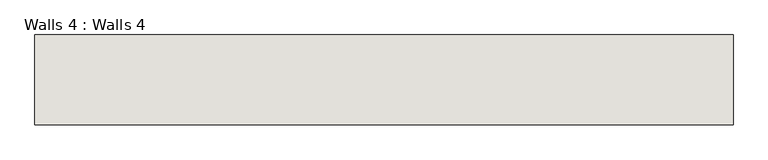
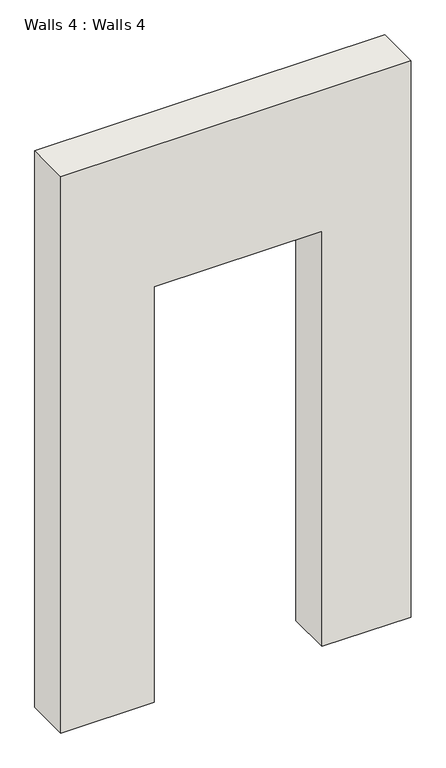
"""IFC4 building model written with IfcOpenShell, lengths in millimetres: wall geometry, Walls 4 : Walls 4."""

from ifc_helpers import new_model, si_unit, frame, origin, place, context, project, spatial, polyline, outline, extrude, source, transform, mapped, element, save


def walls_4_walls_4_cd32183e(model_context):
    return source(origin(), model_context, "Body", "SweptSolid", [
        extrude(outline(polyline([(12109.1166012, -6816.4084212), (12109.1166012, -9490.3075311), (7623.0321664, -9490.3075311), (7623.0321664, -8777.0745124), (10972.8, -8777.0745124), (10972.8, -7495.2589248), (7623.0321664, -7495.2589248), (7623.0321664, -6816.4084212), (12109.1166012, -6816.4084212)])), frame((0.0, -896.8189974, 0.0), z_axis=(0.0, 1.0, 0.0), x_axis=(0.0, 0.0, 1.0)), (0.0, 0.0, 1.0), 344.5607879),
    ])


if __name__ == "__main__":
    model = new_model("IFC4")
    model_context = context("Model", 3, world=origin())
    ifc_project = project(units=[si_unit("LENGTHUNIT", "METRE", prefix="MILLI")], contexts=[model_context])
    site = spatial("IfcSite", under=ifc_project)
    building = spatial("IfcBuilding", under=site)
    placement = place(None, origin())
    walls_4_walls_4_shape = walls_4_walls_4_cd32183e(model_context)
    element("IfcWall", 1, ObjectType="Walls 4 : Walls 4", at=placement, inside=building, context=model_context, shape_type="MappedRepresentation", body=[
        mapped(walls_4_walls_4_shape, transform((0.0, 0.0, 0.0), x_axis=(1.0, 0.0, 0.0), y_axis=(0.0, 1.0, 0.0), z_axis=(0.0, 0.0, 1.0))),
    ])
    save(model, "model.ifc")

# Revit data of these elements
# Element 1 (IfcWall, "Walls 4 : Walls 4")
#   Materials on its faces: "Default Wall"
# Materials
#   "Default Wall": colour RGB 128 128 128, transparency 0
